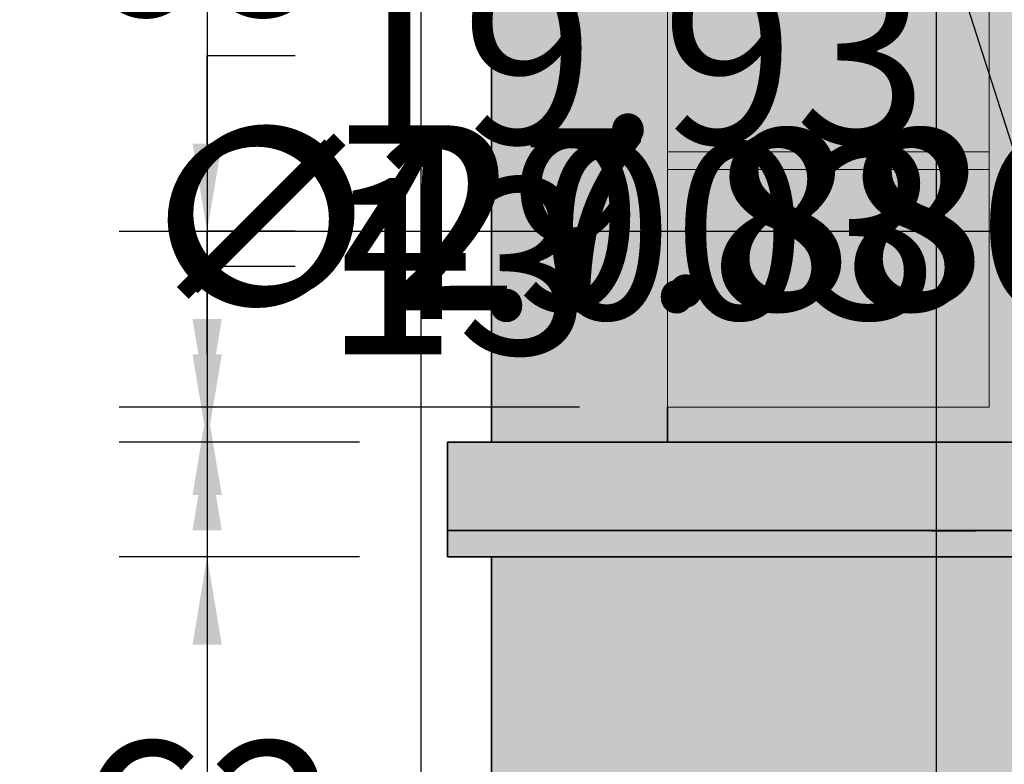
# Model space of a CAD drawing. Units: millimetres. Extents: x 130 to 1021, y 147 to 699.
# Tile 16 of 40: x 254 to 366, y 440 to 525. Entities that reach past the tile are written whole.
import ezdxf

# ---------------------------------------------------------------- set-up
doc = ezdxf.new("R2010")
doc.units = ezdxf.units.MM
doc.header["$MEASUREMENT"] = 0
for name, color, linetype, lineweight in [('A-ANNO-DIMS', 2, 'Continuous', 18), ('A-ELEV', 7, 'Continuous', 35), ('A-ELEV-PATT', 9, 'Continuous', 13), ('A-GLAZ', 4, 'Continuous', 18)]:
    doc.layers.add(name, color=color, linetype=linetype, lineweight=lineweight)
doc.styles.get("Standard").update_dxf_attribs({"font": 'arial.ttf'})
doc.dimstyles.get("Standard").update_dxf_attribs({"dimtxt": 20, "dimasz": 10, "dimexe": 10, "dimexo": 10, "dimgap": 5, "dimtad": 0, "dimtih": 1, "dimtoh": 1, "dimdec": 0, "dimzin": 0, "dimdsep": 46, "dimtxsty": 'Standard', "dimcen": 5, "dimadec": 0, "dimazin": 0, "dimtfac": 1, "dimtdec": 0, "dimtofl": 0, "dimtmove": 0, "dimatfit": 3, "dimfxl": 1, "dimtolj": 1, "dimtzin": 0, "dimarcsym": 0})

# ---------------------------------------------------------------- blocks, each defined once
blk = doc.blocks.new('*D11')
at = {"layer": 'A-ANNO-DIMS', "color": 0, "lineweight": -2, "transparency": 16777216}
for p, q in [((737.37, 648.7), (737.37, 149.74)), ((299.37, 566.95), (299.37, 149.74)), ((309.37, 159.74), (490.86, 159.74)), ((727.37, 159.74), (545.89, 159.74))]:
    blk.add_line(p, q, dxfattribs=at)
at = {"layer": 'A-ANNO-DIMS', "color": 0, "transparency": 16777216}
for points in [[(309.37, 161.41), (309.37, 158.07), (299.37, 159.74)], [(727.37, 161.41), (727.37, 158.07), (737.37, 159.74)]]:
    blk.add_solid(points, dxfattribs=at)
at = {"layer": 'Defpoints', "color": 0, "transparency": 16777216}
for p in [(737.37, 658.7), (299.37, 576.95), (737.37, 159.74)]:
    blk.add_point(p, dxfattribs=at)
at = {"layer": 'A-ANNO-DIMS', "color": 0, "transparency": 16777216, "insert": (518.37, 159.74), "char_height": 20, "attachment_point": 5}
blk.add_mtext('\\A1;438', dxfattribs=at)
blk = doc.blocks.new('*D12')
at = {"layer": 'A-ANNO-DIMS', "color": 0, "lineweight": -2, "transparency": 16777216}
for p, q in [((477.37, 661.95), (265.07, 661.95)), ((275.07, 651.95), (275.07, 438.2)), ((275.07, 194.04), (275.07, 407.78)), ((357.16, 184.04), (265.07, 184.04))]:
    blk.add_line(p, q, dxfattribs=at)
at = {"layer": 'A-ANNO-DIMS', "color": 0, "transparency": 16777216}
for points in [[(273.41, 651.95), (276.74, 651.95), (275.07, 661.95)], [(273.41, 194.04), (276.74, 194.04), (275.07, 184.04)]]:
    blk.add_solid(points, dxfattribs=at)
at = {"layer": 'Defpoints', "color": 0, "transparency": 16777216}
for p in [(275.07, 661.95), (487.37, 661.95), (367.16, 184.04)]:
    blk.add_point(p, dxfattribs=at)
at = {"layer": 'A-ANNO-DIMS', "color": 0, "transparency": 16777216, "insert": (275.07, 422.99), "char_height": 20, "attachment_point": 5}
blk.add_mtext('\\A1;477.9', dxfattribs=at)
blk = doc.blocks.new('*D15')
at = {"layer": 'A-ANNO-DIMS', "color": 0, "lineweight": -2, "transparency": 16777216}
for p, q in [((327.37, 579.88), (327.37, 696.25)), ((357.94, 411.95), (357.94, 696.25)), ((337.37, 686.25), (347.94, 686.25)), ((357.94, 686.25), (367.94, 686.25))]:
    blk.add_line(p, q, dxfattribs=at)
at = {"layer": 'A-ANNO-DIMS', "color": 0, "transparency": 16777216}
for points in [[(337.37, 687.91), (337.37, 684.58), (327.37, 686.25)], [(347.94, 687.91), (347.94, 684.58), (357.94, 686.25)]]:
    blk.add_solid(points, dxfattribs=at)
at = {"layer": 'Defpoints', "color": 0, "transparency": 16777216}
for p in [(357.94, 686.25), (327.37, 569.88), (357.94, 401.95)]:
    blk.add_point(p, dxfattribs=at)
at = {"layer": 'A-ANNO-DIMS', "color": 0, "transparency": 16777216, "insert": (406.68, 686.25), "char_height": 20, "attachment_point": 5}
blk.add_mtext('\\A1;30.57', dxfattribs=at)
blk = doc.blocks.new('*D16')
at = {"layer": 'A-ANNO-DIMS', "color": 0, "lineweight": -2, "transparency": 16777216}
for p, q in [((357.94, 411.95), (357.94, 696.25)), ((363.92, 579.88), (363.92, 696.25)), ((347.94, 686.25), (337.94, 686.25)), ((373.92, 686.25), (383.92, 686.25))]:
    blk.add_line(p, q, dxfattribs=at)
at = {"layer": 'A-ANNO-DIMS', "color": 0, "transparency": 16777216}
for points in [[(347.94, 687.91), (347.94, 684.58), (357.94, 686.25)], [(373.92, 687.91), (373.92, 684.58), (363.92, 686.25)]]:
    blk.add_solid(points, dxfattribs=at)
at = {"layer": 'Defpoints', "color": 0, "transparency": 16777216}
for p in [(363.92, 686.25), (363.92, 569.88), (357.94, 401.95)]:
    blk.add_point(p, dxfattribs=at)
at = {"layer": 'A-ANNO-DIMS', "color": 0, "transparency": 16777216, "insert": (420.74, 686.25), "char_height": 20, "attachment_point": 5}
blk.add_mtext('\\A1;5.981', dxfattribs=at)
blk = doc.blocks.new('*D17')
at = {"layer": 'A-ANNO-DIMS', "color": 0, "lineweight": -2, "transparency": 16777216}
for p, q in [((363.92, 579.88), (363.92, 696.25)), ((375.85, 490.22), (375.85, 696.25)), ((353.92, 686.25), (343.92, 686.25)), ((385.85, 686.25), (395.85, 686.25))]:
    blk.add_line(p, q, dxfattribs=at)
at = {"layer": 'A-ANNO-DIMS', "color": 0, "transparency": 16777216}
for points in [[(353.92, 687.91), (353.92, 684.58), (363.92, 686.25)], [(385.85, 687.91), (385.85, 684.58), (375.85, 686.25)]]:
    blk.add_solid(points, dxfattribs=at)
at = {"layer": 'Defpoints', "color": 0, "transparency": 16777216}
for p in [(375.85, 686.25), (363.92, 569.88), (375.85, 480.22)]:
    blk.add_point(p, dxfattribs=at)
at = {"layer": 'A-ANNO-DIMS', "color": 0, "transparency": 16777216, "insert": (441.44, 686.25), "char_height": 20, "attachment_point": 5}
blk.add_mtext('\\A1;11.928', dxfattribs=at)
blk = doc.blocks.new('*D18')
at = {"layer": 'A-ANNO-DIMS', "color": 0, "lineweight": -2, "transparency": 16777216}
for p, q in [((375.85, 490.22), (375.85, 696.25)), ((382.37, 388.95), (382.37, 696.25)), ((365.85, 686.25), (355.85, 686.25)), ((392.37, 686.25), (402.37, 686.25))]:
    blk.add_line(p, q, dxfattribs=at)
at = {"layer": 'A-ANNO-DIMS', "color": 0, "transparency": 16777216}
for points in [[(365.85, 687.91), (365.85, 684.58), (375.85, 686.25)], [(392.37, 687.91), (392.37, 684.58), (382.37, 686.25)]]:
    blk.add_solid(points, dxfattribs=at)
at = {"layer": 'Defpoints', "color": 0, "transparency": 16777216}
for p in [(382.37, 686.25), (375.85, 480.22), (382.37, 378.95)]:
    blk.add_point(p, dxfattribs=at)
at = {"layer": 'A-ANNO-DIMS', "color": 0, "transparency": 16777216, "insert": (441.13, 686.25), "char_height": 20, "attachment_point": 5}
blk.add_mtext('\\A1;6.524', dxfattribs=at)
blk = doc.blocks.new('*D40')
at = {"layer": 'A-ANNO-DIMS', "color": 0, "lineweight": -2, "transparency": 16777216}
for p, q in [((292.37, 463.95), (265.07, 463.95)), ((275.07, 453.95), (275.07, 448.16)), ((275.07, 411.95), (275.07, 417.74)), ((297.37, 401.95), (265.07, 401.95))]:
    blk.add_line(p, q, dxfattribs=at)
at = {"layer": 'A-ANNO-DIMS', "color": 0, "transparency": 16777216}
for points in [[(273.41, 453.95), (276.74, 453.95), (275.07, 463.95)], [(273.41, 411.95), (276.74, 411.95), (275.07, 401.95)]]:
    blk.add_solid(points, dxfattribs=at)
at = {"layer": 'Defpoints', "color": 0, "transparency": 16777216}
for p in [(275.07, 463.95), (302.37, 463.95), (307.37, 401.95)]:
    blk.add_point(p, dxfattribs=at)
at = {"layer": 'A-ANNO-DIMS', "color": 0, "transparency": 16777216, "insert": (275.07, 432.95), "char_height": 20, "attachment_point": 5}
blk.add_mtext('\\A1;62', dxfattribs=at)
blk = doc.blocks.new('*D41')
at = {"layer": 'A-ANNO-DIMS', "color": 0, "lineweight": -2, "transparency": 16777216}
for p, q in [((275.07, 486.95), (275.07, 496.95)), ((275.07, 496.95), (285.07, 496.95)), ((292.37, 476.95), (265.07, 476.95)), ((292.37, 463.95), (265.07, 463.95)), ((275.07, 453.95), (275.07, 443.95))]:
    blk.add_line(p, q, dxfattribs=at)
at = {"layer": 'A-ANNO-DIMS', "color": 0, "transparency": 16777216}
for points in [[(273.41, 486.95), (276.74, 486.95), (275.07, 476.95)], [(273.41, 453.95), (276.74, 453.95), (275.07, 463.95)]]:
    blk.add_solid(points, dxfattribs=at)
at = {"layer": 'Defpoints', "color": 0, "transparency": 16777216}
for p in [(275.07, 476.95), (302.37, 476.95), (302.37, 463.95)]:
    blk.add_point(p, dxfattribs=at)
at = {"layer": 'A-ANNO-DIMS', "color": 0, "transparency": 16777216, "insert": (303.46, 496.95), "char_height": 20, "attachment_point": 5}
blk.add_mtext('\\A1;13', dxfattribs=at)
blk = doc.blocks.new('*D42')
at = {"layer": 'A-ANNO-DIMS', "color": 0, "lineweight": -2, "transparency": 16777216}
for p, q in [((275.07, 490.95), (275.07, 500.95)), ((275.07, 500.95), (285.07, 500.95)), ((317.37, 480.95), (265.07, 480.95)), ((292.37, 476.95), (265.07, 476.95)), ((275.07, 466.95), (275.07, 456.95))]:
    blk.add_line(p, q, dxfattribs=at)
at = {"layer": 'A-ANNO-DIMS', "color": 0, "transparency": 16777216}
for points in [[(273.41, 490.95), (276.74, 490.95), (275.07, 480.95)], [(273.41, 466.95), (276.74, 466.95), (275.07, 476.95)]]:
    blk.add_solid(points, dxfattribs=at)
at = {"layer": 'Defpoints', "color": 0, "transparency": 16777216}
for p in [(275.07, 480.95), (327.37, 480.95), (302.37, 476.95)]:
    blk.add_point(p, dxfattribs=at)
at = {"layer": 'A-ANNO-DIMS', "color": 0, "transparency": 16777216, "insert": (324.22, 500.95), "char_height": 20, "attachment_point": 5}
blk.add_mtext('\\A1;4.003', dxfattribs=at)
blk = doc.blocks.new('*D43')
at = {"layer": 'A-ANNO-DIMS', "color": 0, "lineweight": -2, "transparency": 16777216}
for p, q in [((275.07, 510.88), (275.07, 520.88)), ((275.07, 520.88), (285.07, 520.88)), ((404.65, 500.88), (265.07, 500.88)), ((317.37, 480.95), (265.07, 480.95)), ((275.07, 470.95), (275.07, 460.95))]:
    blk.add_line(p, q, dxfattribs=at)
at = {"layer": 'A-ANNO-DIMS', "color": 0, "transparency": 16777216}
for points in [[(273.41, 510.88), (276.74, 510.88), (275.07, 500.88)], [(273.41, 470.95), (276.74, 470.95), (275.07, 480.95)]]:
    blk.add_solid(points, dxfattribs=at)
at = {"layer": 'Defpoints', "color": 0, "transparency": 16777216}
for p in [(275.07, 500.88), (414.65, 500.88), (327.37, 480.95)]:
    blk.add_point(p, dxfattribs=at)
at = {"layer": 'A-ANNO-DIMS', "color": 0, "transparency": 16777216, "insert": (322.88, 520.88), "char_height": 20, "attachment_point": 5}
blk.add_mtext('\\A1;19.93', dxfattribs=at)
blk = doc.blocks.new('*D44')
at = {"layer": 'A-ANNO-DIMS', "color": 0, "lineweight": -2, "transparency": 16777216}
for p, q in [((317.37, 569.88), (265.07, 569.88)), ((275.07, 559.88), (275.07, 550.59)), ((275.07, 510.88), (275.07, 520.17)), ((404.65, 500.88), (265.07, 500.88))]:
    blk.add_line(p, q, dxfattribs=at)
at = {"layer": 'A-ANNO-DIMS', "color": 0, "transparency": 16777216}
for points in [[(273.41, 559.88), (276.74, 559.88), (275.07, 569.88)], [(273.41, 510.88), (276.74, 510.88), (275.07, 500.88)]]:
    blk.add_solid(points, dxfattribs=at)
at = {"layer": 'Defpoints', "color": 0, "transparency": 16777216}
for p in [(275.07, 569.88), (327.37, 569.88), (414.65, 500.88)]:
    blk.add_point(p, dxfattribs=at)
at = {"layer": 'A-ANNO-DIMS', "color": 0, "transparency": 16777216, "insert": (275.07, 535.38), "char_height": 20, "attachment_point": 5}
blk.add_mtext('\\A1;69', dxfattribs=at)
blk = doc.blocks.new('*D62')
at = {"layer": 'A-ANNO-DIMS', "color": 0, "lineweight": -2, "transparency": 16777216}
for p, q in [((414.65, 495.88), (414.65, 505.88)), ((379.73, 501.93), (389.72, 501.63)), ((409.65, 500.88), (419.65, 500.88))]:
    blk.add_line(p, q, dxfattribs=at)
at = {"layer": 'A-ANNO-DIMS', "color": 0, "transparency": 16777216}
blk.add_solid([(389.77, 503.29), (389.67, 499.96), (399.72, 501.33)], dxfattribs=at)
at = {"layer": 'Defpoints', "color": 0, "transparency": 16777216}
for p in [(399.72, 501.33), (429.59, 500.43)]:
    blk.add_point(p, dxfattribs=at)
at = {"layer": 'A-ANNO-DIMS', "color": 0, "transparency": 16777216, "insert": (322.34, 501.93), "char_height": 20, "attachment_point": 5}
blk.add_mtext('\\A1;∅29.886', dxfattribs=at)
blk = doc.blocks.new('*D63')
at = {"layer": 'A-ANNO-DIMS', "color": 0, "lineweight": -2, "transparency": 16777216}
for p, q in [((414.65, 495.88), (414.65, 505.88)), ((380.75, 502.59), (390.74, 502.09)), ((409.65, 500.88), (419.65, 500.88))]:
    blk.add_line(p, q, dxfattribs=at)
at = {"layer": 'A-ANNO-DIMS', "color": 0, "transparency": 16777216}
blk.add_solid([(390.82, 503.75), (390.66, 500.42), (400.73, 501.58)], dxfattribs=at)
at = {"layer": 'Defpoints', "color": 0, "transparency": 16777216}
for p in [(400.73, 501.58), (428.58, 500.18)]:
    blk.add_point(p, dxfattribs=at)
at = {"layer": 'A-ANNO-DIMS', "color": 0, "transparency": 16777216, "insert": (323.37, 502.59), "char_height": 20, "attachment_point": 5}
blk.add_mtext('\\A1;∅27.886', dxfattribs=at)
blk = doc.blocks.new('*D64')
at = {"layer": 'A-ANNO-DIMS', "color": 0, "lineweight": -2, "transparency": 16777216}
for p, q in [((502.05, 450.93), (502.05, 460.93)), ((497.05, 455.93), (507.05, 455.93)), ((363.96, 263.06), (409.92, 327.25)), ((353.96, 263.06), (363.96, 263.06))]:
    blk.add_line(p, q, dxfattribs=at)
at = {"layer": 'A-ANNO-DIMS', "color": 0, "transparency": 16777216}
blk.add_solid([(408.57, 328.22), (411.28, 326.28), (415.74, 335.39)], dxfattribs=at)
at = {"layer": 'Defpoints', "color": 0, "transparency": 16777216}
for p in [(502.05, 455.93), (415.74, 335.39)]:
    blk.add_point(p, dxfattribs=at)
at = {"layer": 'A-ANNO-DIMS', "color": 0, "transparency": 16777216, "insert": (297.8, 263.06), "char_height": 20, "attachment_point": 5}
blk.add_mtext('\\A1;R148.25', dxfattribs=at)
blk = doc.blocks.new('*D66')
at = {"layer": 'A-ANNO-DIMS', "color": 0, "lineweight": -2, "transparency": 16777216}
for p, q in [((341.58, 557.19), (351.58, 557.19)), ((351.58, 557.19), (376.95, 478.14)), ((427.37, 315.98), (427.37, 325.98)), ((422.37, 320.98), (432.37, 320.98))]:
    blk.add_line(p, q, dxfattribs=at)
at = {"layer": 'A-ANNO-DIMS', "color": 0, "transparency": 16777216}
blk.add_solid([(378.53, 478.64), (375.36, 477.63), (380, 468.61)], dxfattribs=at)
at = {"layer": 'Defpoints', "color": 0, "transparency": 16777216}
for p in [(380, 468.61), (427.37, 320.98)]:
    blk.add_point(p, dxfattribs=at)
at = {"layer": 'A-ANNO-DIMS', "color": 0, "transparency": 16777216, "insert": (263.53, 557.19), "char_height": 20, "attachment_point": 5}
blk.add_mtext('\\A1;4X R155.05', dxfattribs=at)
blk = doc.blocks.new('*D68')
at = {"layer": 'A-ANNO-DIMS', "color": 0, "lineweight": -2, "transparency": 16777216}
for p, q in [((361.84, 579.76), (371.84, 579.76)), ((371.84, 579.76), (392.17, 506.69)), ((433.19, 354.23), (433.19, 364.23)), ((428.19, 359.23), (438.19, 359.23))]:
    blk.add_line(p, q, dxfattribs=at)
at = {"layer": 'A-ANNO-DIMS', "color": 0, "transparency": 16777216}
blk.add_solid([(393.77, 507.14), (390.56, 506.25), (394.85, 497.06)], dxfattribs=at)
at = {"layer": 'Defpoints', "color": 0, "transparency": 16777216}
for p in [(394.85, 497.06), (433.19, 359.23)]:
    blk.add_point(p, dxfattribs=at)
at = {"layer": 'A-ANNO-DIMS', "color": 0, "transparency": 16777216, "insert": (305.76, 579.76), "char_height": 20, "attachment_point": 5}
blk.add_mtext('\\A1;R143.06', dxfattribs=at)
blk = doc.blocks.new('*D70')
at = {"layer": 'A-ANNO-DIMS', "color": 0, "lineweight": -2, "transparency": 16777216}
for p, q in [((370.14, 588.4), (380.14, 588.4)), ((380.14, 588.4), (397.47, 517.01)), ((432.65, 367.11), (432.65, 377.11)), ((427.65, 372.11), (437.65, 372.11))]:
    blk.add_line(p, q, dxfattribs=at)
at = {"layer": 'A-ANNO-DIMS', "color": 0, "transparency": 16777216}
blk.add_solid([(399.09, 517.4), (395.85, 516.62), (399.83, 507.29)], dxfattribs=at)
at = {"layer": 'Defpoints', "color": 0, "transparency": 16777216}
for p in [(399.83, 507.29), (432.65, 372.11)]:
    blk.add_point(p, dxfattribs=at)
at = {"layer": 'A-ANNO-DIMS', "color": 0, "transparency": 16777216, "insert": (323.76, 588.4), "char_height": 20, "attachment_point": 5}
blk.add_mtext('\\A1;R139.1', dxfattribs=at)
blk = doc.blocks.new('*D73')
at = {"layer": 'A-ANNO-DIMS', "color": 0, "lineweight": -2, "transparency": 16777216}
for p, q in [((402.68, 571.45), (412.68, 571.45)), ((412.68, 571.45), (419.05, 502.17)), ((432.11, 355.14), (432.11, 365.14)), ((427.11, 360.14), (437.11, 360.14))]:
    blk.add_line(p, q, dxfattribs=at)
at = {"layer": 'A-ANNO-DIMS', "color": 0, "transparency": 16777216}
blk.add_solid([(420.71, 502.32), (417.39, 502.01), (419.97, 492.21)], dxfattribs=at)
at = {"layer": 'Defpoints', "color": 0, "transparency": 16777216}
for p in [(419.97, 492.21), (432.11, 360.14)]:
    blk.add_point(p, dxfattribs=at)
at = {"layer": 'A-ANNO-DIMS', "color": 0, "transparency": 16777216, "insert": (346.7, 571.45), "char_height": 20, "attachment_point": 5}
blk.add_mtext('\\A1;R132.62', dxfattribs=at)

msp = doc.modelspace()

# ---------------------------------------------------------------- hatches: boundary and pattern name
at = {"layer": 'A-ELEV-PATT'}
h = msp.add_hatch(color=256, dxfattribs=at)
h.dxf.hatch_style = 1
h.paths.add_polyline_path([(737.3738, 658.6988, 0.01359606), (632.4019, 661.9473), (607.3738, 661.9473), (487.3738, 661.9473), (487.3738, 649.9473), (607.3738, 649.9473), (632.3794, 649.9473, -0.01368411), (737.3738, 646.6784)])
h.paths.add_polyline_path([(732.3738, 643.9599, 0.01305286), (632.3738, 646.9473), (607.3738, 646.9473), (487.3738, 646.9473), (487.3738, 596.9473), (632.3738, 596.9473, -0.01305286), (732.3738, 593.9599)])
h.paths.add_polyline_path([(737.3738, 593.6732, 0.01370629), (632.3738, 596.9473), (487.3738, 596.9473), (487.3738, 586.9473), (632.355, 586.9473, -0.01378075), (737.3738, 583.6559)])
h.paths.add_polyline_path([(447.3738, 646.9473), (307.3738, 646.9473), (302.3738, 646.9473), (302.3738, 634.9473), (447.3738, 634.9473)])
h.paths.add_polyline_path([(447.3738, 631.9473), (307.3738, 631.9473), (307.3738, 586.9473), (447.3738, 586.9473)])
h.paths.add_polyline_path([(447.3738, 586.9473), (307.3738, 586.9473), (302.3738, 586.9473), (302.3738, 576.9473), (447.3738, 576.9473)])
h.paths.add_polyline_path([(447.3738, 573.9473), (367.3738, 573.9473), (367.3738, 539.9473), (447.3738, 539.9473)])
h.paths.add_polyline_path([(447.3738, 537.9473), (367.3738, 537.9473), (367.3738, 507.9473), (400.392, 507.4253, -0.00172798), (401.3281, 507.6451, -0.52200255), (425.6117, 511.0391, -0.03918489), (447.3738, 510.4359), (447.3738, 510.7883)])
h.paths.add_polyline_path([(394.7238, 505.9473), (367.3738, 505.9473), (367.3738, 476.9473, -0.0146512), (375.8501, 480.2159), (376.1506, 499.2266, -0.03554194)])
h.paths.add_polyline_path([(632.3738, 583.9473), (552.3738, 583.9473), (552.3738, 550.9473), (632.3738, 550.9473)])
h.paths.add_polyline_path([(632.3738, 548.9473), (552.3738, 548.9473), (552.3738, 515.9473), (632.3738, 515.9473)])
h.paths.add_polyline_path([(632.3738, 513.9473), (552.3738, 513.9473), (552.3738, 476.9473), (632.3738, 476.9473)])
h.paths.add_polyline_path([(737.3738, 473.6903, 0.01363261), (632.3926, 476.9473), (552.3738, 476.9473), (487.3738, 476.9473), (487.3738, 466.9473), (632.3738, 466.9473, -0.01370629), (737.3738, 463.6732)])
h.paths.add_polyline_path([(732.3738, 460.9552, 0.01307409), (632.3681, 463.9473), (487.3738, 463.9473), (487.3738, 407.735, -0.00322862), (489.3544, 406.9473), (632.3926, 406.9473, -0.01298259), (732.3738, 403.9755)])
h.paths.add_polyline_path([(487.3738, 463.9473, 0.20132998), (367.3738, 463.9473), (367.3738, 407.735, -0.18820307), (487.3738, 407.735)])
h.paths.add_polyline_path([(367.3738, 476.9473), (367.3738, 466.9473, -0.20133085), (487.3738, 466.9473), (487.3738, 476.9473, 0.20132998)])
h.paths.add_polyline_path([(367.3738, 463.9473), (307.3738, 463.9473), (307.3738, 401.9473), (357.9413, 401.9473), (367.3738, 407.735)])
h.paths.add_polyline_path([(367.3738, 476.9473), (302.3738, 476.9473), (302.3738, 466.9473), (367.3738, 466.9473)])
h.paths.add_polyline_path([(632.8184, 366.9453), (552.3738, 366.9453), (552.3738, 393.9473), (632.8184, 393.9473)])
h.paths.add_polyline_path([(632.8184, 357.2114), (632.8184, 363.9453), (552.3738, 363.9453), (552.3738, 357.2114), (552.3738, 336.9453), (632.8184, 336.9453)])
h.paths.add_polyline_path([(632.8184, 333.9453), (552.3738, 333.9453), (552.3738, 306.9453), (632.8184, 306.9453)])
h.paths.add_polyline_path([(632.8184, 303.9453), (552.3738, 303.9453), (552.3738, 273.9473), (632.355, 273.9473, 0.00006077), (632.8184, 273.9491)])
h.paths.add_polyline_path([(737.3738, 403.6903, 0.01363261), (632.3926, 406.9473), (489.3544, 406.9473, 0.19154808), (367.3738, 407.735), (367.3738, 396.9473, -0.20133085), (487.3738, 396.9473), (632.3738, 396.9473, -0.01370629), (737.3738, 393.6732)])
h.paths.add_polyline_path([(357.9413, 401.9473), (307.3738, 401.9473), (307.3738, 391.9473), (357.9413, 391.9473)])
h.paths.add_polyline_path([(357.9413, 357.2114), (357.9413, 388.9473), (307.3738, 388.9473), (307.3738, 357.2114), (307.3738, 273.9473), (357.9413, 273.9473)])
h.paths.add_polyline_path([(732.3738, 263.93, -0.0130317), (632.3794, 260.9473), (466.7667, 260.9473), (466.7667, 240.9473), (469.8406, 236.978), (469.8406, 221.978), (472.9145, 218.0087), (472.9145, 213.9473), (607.3738, 213.9473), (732.3738, 213.9473)])
h.paths.add_polyline_path([(732.3738, 290.889), (722.479, 290.889), (722.479, 301.889), (732.3738, 301.889), (732.3738, 305.889), (722.479, 305.889), (722.479, 316.889), (732.3738, 316.889), (732.3738, 320.889), (722.479, 320.889), (722.479, 331.889), (732.3738, 331.889), (732.3738, 335.889), (722.479, 335.889), (722.479, 346.889), (732.3738, 346.889), (732.3738, 350.889), (722.479, 350.889), (722.479, 361.889), (732.3738, 361.889), (732.3738, 365.889), (722.479, 365.889), (722.479, 376.889), (732.3738, 376.889), (732.3738, 380.889), (722.479, 380.889), (722.479, 391.4848, 0.00052326), (718.479, 391.6843), (718.479, 380.889), (707.479, 380.889), (707.479, 392.1896, 0.00052307), (703.479, 392.3576), (703.479, 380.889), (692.479, 380.889), (692.479, 392.7765, 0.00052292), (688.479, 392.9131), (688.479, 380.889), (677.479, 380.889), (677.479, 393.2456, 0.00052279), (673.479, 393.3508), (673.479, 380.889), (662.479, 380.889), (662.479, 393.597, 0.0005227), (658.479, 393.6709), (658.479, 380.889), (647.479, 380.889), (647.479, 393.8308, 0.00052264), (643.479, 393.8732), (643.479, 380.889), (632.8184, 380.889), (632.8184, 376.889), (643.479, 376.889), (643.479, 365.889), (632.8184, 365.889), (632.8184, 361.889), (643.479, 361.889), (643.479, 350.889), (632.8184, 350.889), (632.8184, 346.889), (643.479, 346.889), (643.479, 335.889), (632.8184, 335.889), (632.8184, 331.889), (643.479, 331.889), (643.479, 320.889), (632.8184, 320.889), (632.8184, 316.889), (643.479, 316.889), (643.479, 305.889), (632.8184, 305.889), (632.8184, 301.889), (643.479, 301.889), (643.479, 290.889), (632.8184, 290.889), (632.8184, 286.889), (643.479, 286.889), (643.479, 274.0217, 0.00052456), (647.479, 274.0643), (647.479, 286.889), (658.479, 286.889), (658.479, 274.2248, 0.00052462), (662.479, 274.2989), (662.479, 286.889), (673.479, 286.889), (673.479, 274.546, 0.00052471), (677.479, 274.6516), (677.479, 286.889), (688.479, 286.889), (688.479, 274.9853, 0.00052484), (692.479, 275.1224), (692.479, 286.889), (703.479, 286.889), (703.479, 275.5429, 0.000525), (707.479, 275.7115), (707.479, 286.889), (718.479, 286.889), (718.479, 276.2187, 0.00052519), (722.479, 276.4189), (722.479, 286.889), (732.3738, 286.889)])
h.paths.add_polyline_path([(718.479, 290.889), (707.479, 290.889), (707.479, 301.889), (718.479, 301.889)], flags=16)
h.paths.add_polyline_path([(703.479, 290.889), (692.479, 290.889), (692.479, 301.889), (703.479, 301.889)], flags=16)
h.paths.add_polyline_path([(718.479, 305.889), (707.479, 305.889), (707.479, 316.889), (718.479, 316.889)], flags=16)
h.paths.add_polyline_path([(703.479, 305.889), (692.479, 305.889), (692.479, 316.889), (703.479, 316.889)], flags=16)
h.paths.add_polyline_path([(688.479, 290.889), (677.479, 290.889), (677.479, 301.889), (688.479, 301.889)], flags=16)
h.paths.add_polyline_path([(718.479, 320.889), (707.479, 320.889), (707.479, 331.889), (718.479, 331.889)], flags=16)
h.paths.add_polyline_path([(688.479, 305.889), (677.479, 305.889), (677.479, 316.889), (688.479, 316.889)], flags=16)
h.paths.add_polyline_path([(703.479, 320.889), (692.479, 320.889), (692.479, 331.889), (703.479, 331.889)], flags=16)
h.paths.add_polyline_path([(688.479, 320.889), (677.479, 320.889), (677.479, 331.889), (688.479, 331.889)], flags=16)
h.paths.add_polyline_path([(673.479, 290.889), (662.479, 290.889), (662.479, 301.889), (673.479, 301.889)], flags=16)
h.paths.add_polyline_path([(718.479, 335.889), (707.479, 335.889), (707.479, 346.889), (718.479, 346.889)], flags=16)
h.paths.add_polyline_path([(673.479, 305.889), (662.479, 305.889), (662.479, 316.889), (673.479, 316.889)], flags=16)
h.paths.add_polyline_path([(703.479, 335.889), (692.479, 335.889), (692.479, 346.889), (703.479, 346.889)], flags=16)
h.paths.add_polyline_path([(673.479, 320.889), (662.479, 320.889), (662.479, 331.889), (673.479, 331.889)], flags=16)
h.paths.add_polyline_path([(688.479, 335.889), (677.479, 335.889), (677.479, 346.889), (688.479, 346.889)], flags=16)
h.paths.add_polyline_path([(658.479, 290.889), (647.479, 290.889), (647.479, 301.889), (658.479, 301.889)], flags=16)
h.paths.add_polyline_path([(718.479, 350.889), (707.479, 350.889), (707.479, 361.889), (718.479, 361.889)], flags=16)
h.paths.add_polyline_path([(658.479, 305.889), (647.479, 305.889), (647.479, 316.889), (658.479, 316.889)], flags=16)
h.paths.add_polyline_path([(703.479, 350.889), (692.479, 350.889), (692.479, 361.889), (703.479, 361.889)], flags=16)
h.paths.add_polyline_path([(673.479, 335.889), (662.479, 335.889), (662.479, 346.889), (673.479, 346.889)], flags=16)
h.paths.add_polyline_path([(658.479, 320.889), (647.479, 320.889), (647.479, 331.889), (658.479, 331.889)], flags=16)
h.paths.add_polyline_path([(688.479, 350.889), (677.479, 350.889), (677.479, 361.889), (688.479, 361.889)], flags=16)
h.paths.add_polyline_path([(718.479, 365.889), (707.479, 365.889), (707.479, 376.889), (718.479, 376.889)], flags=16)
h.paths.add_polyline_path([(658.479, 335.889), (647.479, 335.889), (647.479, 346.889), (658.479, 346.889)], flags=16)
h.paths.add_polyline_path([(673.479, 350.889), (662.479, 350.889), (662.479, 361.889), (673.479, 361.889)], flags=16)
h.paths.add_polyline_path([(703.479, 365.889), (692.479, 365.889), (692.479, 376.889), (703.479, 376.889)], flags=16)
h.paths.add_polyline_path([(688.479, 365.889), (677.479, 365.889), (677.479, 376.889), (688.479, 376.889)], flags=16)
h.paths.add_polyline_path([(658.479, 350.889), (647.479, 350.889), (647.479, 361.889), (658.479, 361.889)], flags=16)
h.paths.add_polyline_path([(673.479, 365.889), (662.479, 365.889), (662.479, 376.889), (673.479, 376.889)], flags=16)
h.paths.add_polyline_path([(658.479, 365.889), (647.479, 365.889), (647.479, 376.889), (658.479, 376.889)], flags=16)
h.paths.add_polyline_path([(732.3738, 503.9786), (722.3392, 503.9786), (722.3392, 514.9786), (732.3738, 514.9786), (732.3738, 518.9786), (722.3392, 518.9786), (722.3392, 529.9786), (732.3738, 529.9786), (732.3738, 533.9786), (722.3392, 533.9786), (722.3392, 544.9786), (732.3738, 544.9786), (732.3738, 546.9473), (732.3738, 548.9786), (722.3392, 548.9786), (722.3392, 559.9786), (732.3738, 559.9786), (732.3738, 563.9786), (722.3392, 563.9786), (722.3392, 574.9786), (732.3738, 574.9786), (732.3738, 578.9786), (722.3392, 578.9786), (722.3392, 581.4789, 0.00052601), (718.3392, 581.6791), (718.3392, 578.9786), (707.3392, 578.9786), (707.3392, 582.1863, 0.00052582), (703.3392, 582.355), (703.3392, 578.9786), (692.3392, 578.9786), (692.3392, 582.7752, 0.00052566), (688.3392, 582.9123), (688.3392, 578.9786), (677.3392, 578.9786), (677.3392, 583.2457, 0.00052554), (673.3392, 583.3512), (673.3392, 578.9786), (662.3392, 578.9786), (662.3392, 583.5978, 0.00052545), (658.3392, 583.6718), (658.3392, 578.9786), (647.3392, 578.9786), (647.3392, 583.8317, 0.00052539), (643.3392, 583.8741), (643.3392, 578.9786), (632.3738, 578.9786), (632.3738, 574.9786), (643.3392, 574.9786), (643.3392, 563.9786), (632.3738, 563.9786), (632.3738, 559.9786), (643.3392, 559.9786), (643.3392, 548.9786), (632.3738, 548.9786), (632.3738, 544.9786), (643.3392, 544.9786), (643.3392, 533.9786), (632.3738, 533.9786), (632.3738, 529.9786), (643.3392, 529.9786), (643.3392, 518.9786), (632.3738, 518.9786), (632.3738, 515.9473), (632.3738, 514.9786), (643.3392, 514.9786), (643.3392, 503.9786), (632.3738, 503.9786), (632.3738, 499.9786), (643.3392, 499.9786), (643.3392, 488.9786), (632.3738, 488.9786), (632.3738, 484.9786), (643.3392, 484.9786), (643.3392, 476.8751, -0.00051911), (647.3392, 476.8332), (647.3392, 484.9786), (658.3392, 484.9786), (658.3392, 476.6752, -0.00051917), (662.3392, 476.6022), (662.3392, 484.9786), (673.3392, 484.9786), (673.3392, 476.3585, -0.00051926), (677.3392, 476.2543), (677.3392, 484.9786), (688.3392, 484.9786), (688.3392, 475.9248, -0.00051938), (692.3392, 475.7894), (692.3392, 484.9786), (703.3392, 484.9786), (703.3392, 475.3741, -0.00051953), (707.3392, 475.2075), (707.3392, 484.9786), (718.3392, 484.9786), (718.3392, 474.7064, -0.00051972), (722.3392, 474.5086), (722.3392, 484.9786), (732.3738, 484.9786), (732.3738, 488.9786), (722.3392, 488.9786), (722.3392, 499.9786), (732.3738, 499.9786)])
h.paths.add_polyline_path([(718.3392, 503.9786), (707.3392, 503.9786), (707.3392, 514.9786), (718.3392, 514.9786)], flags=16)
h.paths.add_polyline_path([(718.3392, 499.9786), (718.3392, 488.9786), (707.3392, 488.9786), (707.3392, 499.9786)], flags=16)
h.paths.add_polyline_path([(718.3392, 518.9786), (707.3392, 518.9786), (707.3392, 529.9786), (718.3392, 529.9786)], flags=16)
h.paths.add_polyline_path([(703.3392, 503.9786), (692.3392, 503.9786), (692.3392, 514.9786), (703.3392, 514.9786)], flags=16)
h.paths.add_polyline_path([(703.3392, 499.9786), (703.3392, 488.9786), (692.3392, 488.9786), (692.3392, 499.9786)], flags=16)
h.paths.add_polyline_path([(703.3392, 518.9786), (692.3392, 518.9786), (692.3392, 529.9786), (703.3392, 529.9786)], flags=16)
h.paths.add_polyline_path([(718.3392, 533.9786), (707.3392, 533.9786), (707.3392, 544.9786), (718.3392, 544.9786)], flags=16)
h.paths.add_polyline_path([(688.3392, 503.9786), (677.3392, 503.9786), (677.3392, 514.9786), (688.3392, 514.9786)], flags=16)
h.paths.add_polyline_path([(688.3392, 499.9786), (688.3392, 488.9786), (677.3392, 488.9786), (677.3392, 499.9786)], flags=16)
h.paths.add_polyline_path([(703.3392, 533.9786), (692.3392, 533.9786), (692.3392, 544.9786), (703.3392, 544.9786)], flags=16)
h.paths.add_polyline_path([(688.3392, 518.9786), (677.3392, 518.9786), (677.3392, 529.9786), (688.3392, 529.9786)], flags=16)
h.paths.add_polyline_path([(688.3392, 533.9786), (677.3392, 533.9786), (677.3392, 544.9786), (688.3392, 544.9786)], flags=16)
h.paths.add_polyline_path([(718.3392, 548.9786), (707.3392, 548.9786), (707.3392, 559.9786), (718.3392, 559.9786)], flags=16)
h.paths.add_polyline_path([(673.3392, 503.9786), (662.3392, 503.9786), (662.3392, 514.9786), (673.3392, 514.9786)], flags=16)
h.paths.add_polyline_path([(673.3392, 499.9786), (673.3392, 488.9786), (662.3392, 488.9786), (662.3392, 499.9786)], flags=16)
h.paths.add_polyline_path([(703.3392, 548.9786), (692.3392, 548.9786), (692.3392, 559.9786), (703.3392, 559.9786)], flags=16)
h.paths.add_polyline_path([(673.3392, 518.9786), (662.3392, 518.9786), (662.3392, 529.9786), (673.3392, 529.9786)], flags=16)
h.paths.add_polyline_path([(688.3392, 548.9786), (677.3392, 548.9786), (677.3392, 559.9786), (688.3392, 559.9786)], flags=16)
h.paths.add_polyline_path([(673.3392, 533.9786), (662.3392, 533.9786), (662.3392, 544.9786), (673.3392, 544.9786)], flags=16)
h.paths.add_polyline_path([(718.3392, 563.9786), (707.3392, 563.9786), (707.3392, 574.9786), (718.3392, 574.9786)], flags=16)
h.paths.add_polyline_path([(658.3392, 503.9786), (647.3392, 503.9786), (647.3392, 514.9786), (658.3392, 514.9786)], flags=16)
h.paths.add_polyline_path([(658.3392, 499.9786), (658.3392, 488.9786), (647.3392, 488.9786), (647.3392, 499.9786)], flags=16)
h.paths.add_polyline_path([(703.3392, 563.9786), (692.3392, 563.9786), (692.3392, 574.9786), (703.3392, 574.9786)], flags=16)
h.paths.add_polyline_path([(658.3392, 518.9786), (647.3392, 518.9786), (647.3392, 529.9786), (658.3392, 529.9786)], flags=16)
h.paths.add_polyline_path([(673.3392, 548.9786), (662.3392, 548.9786), (662.3392, 559.9786), (673.3392, 559.9786)], flags=16)
h.paths.add_polyline_path([(688.3392, 563.9786), (677.3392, 563.9786), (677.3392, 574.9786), (688.3392, 574.9786)], flags=16)
h.paths.add_polyline_path([(658.3392, 533.9786), (647.3392, 533.9786), (647.3392, 544.9786), (658.3392, 544.9786)], flags=16)
h.paths.add_polyline_path([(673.3392, 563.9786), (662.3392, 563.9786), (662.3392, 574.9786), (673.3392, 574.9786)], flags=16)
h.paths.add_polyline_path([(658.3392, 548.9786), (647.3392, 548.9786), (647.3392, 559.9786), (658.3392, 559.9786)], flags=16)
h.paths.add_polyline_path([(658.3392, 563.9786), (647.3392, 563.9786), (647.3392, 574.9786), (658.3392, 574.9786)], flags=16)
h = msp.add_hatch(color=256, dxfattribs=at)
h.dxf.hatch_style = 1
h.paths.add_polyline_path([(447.3738, 576.9473), (302.3738, 576.9473), (302.3738, 573.9473), (447.3738, 573.9473)])
h.paths.add_polyline_path([(487.3738, 583.9473), (487.3738, 586.9473), (447.3738, 576.9473), (447.3738, 573.9473)])
h.paths.add_polyline_path([(632.355, 586.9473), (487.3738, 586.9473), (487.3738, 583.9473), (632.3738, 583.9473), (632.3738, 583.9472, -0.01380003), (737.3738, 580.6507), (737.3738, 583.6559, 0.01378075)])
h.paths.add_polyline_path([(367.3738, 466.9473), (302.3738, 466.9473), (302.3738, 463.9473), (367.3738, 463.9473)])
h.paths.add_polyline_path([(487.3738, 463.9473), (487.3738, 466.9473, 0.20133085), (367.3738, 466.9473), (367.3738, 463.9473, -0.20132998)])
h.paths.add_polyline_path([(632.3738, 466.9473), (487.3738, 466.9473), (487.3738, 463.9473), (632.3681, 463.9473, -0.01372855), (737.3738, 460.6681), (737.3738, 463.6732, 0.01370629)])
h.paths.add_polyline_path([(632.3738, 396.9473), (487.3738, 396.9473, 0.20133085), (367.3738, 396.9473), (367.3738, 393.9473, -0.20237172), (486.7667, 393.9473), (632.3681, 393.9473, -0.01372855), (737.3738, 390.6681), (737.3738, 393.6732, 0.01370629)])
h.paths.add_polyline_path([(357.9413, 391.9473), (307.3738, 391.9473), (307.3738, 388.9473), (357.9413, 388.9473)])
h.paths.add_polyline_path([(367.3738, 393.9473), (367.3738, 396.9473), (357.9413, 391.924), (357.9413, 388.9473), (358.058, 388.9473)])
h.paths.add_polyline_path([(737.3738, 264.2162), (737.3738, 267.2214, -0.01370629), (632.3738, 263.9473), (463.7667, 263.9473), (466.7667, 260.9473), (632.3794, 260.9473, 0.01368411)])
h.paths.add_polyline_path([(463.7667, 263.9473), (447.3738, 263.9473), (450.3738, 260.9473), (466.7667, 260.9473)])
h.paths.add_polyline_path([(447.3738, 263.9473), (432.3738, 263.9473), (432.3738, 260.9473), (450.3738, 260.9473)])
h.paths.add_polyline_path([(382.3738, 263.9473), (357.9413, 263.9473), (357.9413, 260.9473), (382.3738, 260.9473)])
h.paths.add_polyline_path([(357.9413, 263.9473), (307.3738, 263.9473), (307.3738, 260.9473), (357.9413, 260.9473)])
h = msp.add_hatch(color=256, dxfattribs=at)
h.paths.add_polyline_path([(327.3738, 569.884), (327.3738, 573.9473), (307.3738, 573.9473), (307.3738, 476.9473), (327.3738, 476.9473), (327.3738, 480.95)])
h.paths.add_polyline_path([(486.7667, 386.2639), (486.7667, 393.9473), (466.7667, 393.9473), (466.7667, 357.2114), (466.7667, 311.9335, 0.03427026), (486.7667, 308.4637)])
h.paths.add_polyline_path([(486.7667, 308.4637, -0.03427026), (466.7667, 311.9335), (466.7667, 273.9473), (486.7667, 273.9473)])
h.paths.add_polyline_path([(389.3738, 351.5473), (396.7693, 351.5473, -0.00702703), (393.8774, 354.5473), (389.3738, 354.5473), (389.3738, 359.5775, -0.01903024), (382.3738, 368.424), (382.3738, 249.5473), (432.3738, 249.5473), (432.3738, 325.067, -0.00576734), (429.3738, 326.709), (429.3738, 257.5473), (426.3738, 257.5473), (426.3738, 328.4428, -0.00592542), (423.3738, 330.272), (423.3738, 315.7473), (389.3738, 315.7473), (389.3738, 332.1473), (420.4552, 332.1473, -0.00895099), (416.0768, 335.1473), (389.3738, 335.1473)])
h.paths.add_polyline_path([(389.3738, 312.7473), (423.3738, 312.7473), (423.3738, 296.3473), (389.3738, 296.3473)], flags=16)
h.paths.add_polyline_path([(389.3738, 293.3473), (423.3738, 293.3473), (423.3738, 276.9473), (389.3738, 276.9473)], flags=16)
h.paths.add_polyline_path([(389.3738, 273.9473), (423.3738, 273.9473), (423.3738, 257.5473), (389.3738, 257.5473)], flags=16)
h.paths.add_polyline_path([(432.3738, 378.9473), (382.3738, 378.9473), (382.3738, 368.424, 0.01903024), (389.3738, 359.5775), (389.3738, 370.9473), (423.3738, 370.9473), (423.3738, 354.5473), (393.8774, 354.5473, 0.00702703), (396.7693, 351.5473), (423.3738, 351.5473), (423.3738, 335.1473), (416.0768, 335.1473, 0.00895099), (420.4552, 332.1473), (423.3738, 332.1473), (423.3738, 330.272, 0.00592542), (426.3738, 328.4428), (426.3738, 370.9473), (429.3738, 370.9473), (429.3738, 326.709, 0.00576734), (432.3738, 325.067)])
h.paths.add_polyline_path([(466.7667, 357.2114), (466.7667, 393.9473), (447.3738, 393.9473), (447.3738, 357.2114), (447.3738, 318.1243, 0.0063261), (450.8779, 316.785), (450.8779, 331.5915), (463.5608, 331.5915), (463.5608, 312.7571, 0.00558197), (466.7667, 311.9335)])
h.paths.add_polyline_path([(450.8779, 334.5915), (450.8779, 360.0915), (463.5608, 360.0915), (463.5608, 334.5915)], flags=16)
h.paths.add_polyline_path([(450.8779, 363.0915), (450.8779, 388.6449), (463.5608, 388.6449), (463.5608, 363.0915)], flags=16)
h.paths.add_polyline_path([(466.7667, 311.9335, -0.00558197), (463.5608, 312.7571), (463.5608, 306.0915), (450.8779, 306.0915), (450.8779, 316.785, -0.0063261), (447.3738, 318.1243), (447.3738, 273.9473), (466.7667, 273.9473)])
h.paths.add_polyline_path([(450.8779, 303.0915), (463.5608, 303.0915), (463.5608, 277.5915), (450.8779, 277.5915)], flags=16)
h.paths.add_polyline_path([(552.3738, 357.2114), (552.3738, 393.9473), (486.7667, 393.9473), (486.7667, 386.2639), (544.6354, 386.2639), (544.6354, 280.6619), (486.7667, 280.6619), (486.7667, 273.9473), (552.3738, 273.9473)])
h.paths.add_polyline_path([(487.3738, 583.9473), (472.3738, 580.1973), (472.3738, 507.0765), (472.3738, 505.4251, -0.00564525), (475.3738, 504.4942), (475.3738, 506.3543), (475.3738, 511.9473), (484.3738, 511.9473), (484.3738, 503.8134), (484.3738, 501.2439, -0.00583574), (487.3738, 500.0015)])
h.paths.add_polyline_path([(484.3738, 578.0434), (484.3738, 548.9473), (475.3738, 548.9473), (475.3738, 575.7934)], flags=16)
h.paths.add_polyline_path([(484.3738, 546.9473), (484.3738, 513.9473), (475.3738, 513.9473), (475.3738, 518.7148), (475.3738, 546.9473)], flags=16)
msp.add_hatch(color=256, dxfattribs=at).paths.add_polyline_path([(327.3738, 573.9473), (327.3738, 569.884), (363.922, 569.884), (363.922, 480.95), (327.3738, 480.95), (327.3738, 476.9473), (367.3738, 476.9473), (367.3738, 573.9473)])
h = msp.add_hatch(color=256, dxfattribs=at)
h.paths.add_polyline_path([(327.3738, 541.9473), (327.3738, 539.9473), (363.922, 539.9473), (363.922, 541.9473)])
h.paths.add_polyline_path([(327.3738, 509.9473), (327.3738, 507.9473), (363.922, 507.9473), (363.922, 509.9473)])
h = msp.add_hatch(color=256, dxfattribs=at)
h.dxf.hatch_style = 1
h.paths.add_polyline_path([(364.0891, 218.0087), (361.0152, 221.978), (361.0152, 236.978), (357.9413, 240.9473), (357.9413, 195.9473), (367.163, 184.0395), (367.163, 199.0395), (364.0891, 203.0087)])
h.paths.add_polyline_path([(502.3738, 537.2685), (502.3738, 513.9473), (547.7773, 513.9473), (547.7773, 537.2685)])
h.paths.add_polyline_path([(502.3738, 511.9473), (502.3738, 481.7432), (547.7773, 481.7432), (547.7773, 511.9473)])
h.paths.add_polyline_path([(327.3738, 529.7), (327.3738, 509.9473), (363.922, 509.9473), (363.922, 529.7)])
h.paths.add_polyline_path([(327.3738, 507.9473), (327.3738, 480.95), (363.922, 480.95), (363.922, 507.9473)])

# ---------------------------------------------------------------- linework, layer by layer
at = {"layer": 'A-ELEV'}
for p, q in [((307.3738, 573.9473), (307.3738, 476.9473)), ((327.3738, 480.95), (327.3738, 476.9473)), ((302.3738, 476.9473), (302.3738, 463.9473)), ((367.3738, 476.9473), (302.3738, 476.9473)), ((367.3738, 466.9473), (302.3738, 466.9473)), ((367.3738, 466.9473), (357.3742, 466.8599)), ((367.3738, 463.9473), (302.3738, 463.9473)), ((307.3738, 463.9473), (307.3738, 357.2114))]:
    msp.add_line(p, q, dxfattribs=at)
at = {"layer": 'A-GLAZ'}
for p, q in [((363.922, 509.9473), (327.3738, 509.9473)), ((363.922, 507.9473), (327.3738, 507.9473))]:
    msp.add_line(p, q, dxfattribs=at)
msp.add_lwpolyline([(363.922, 569.884), (327.3738, 569.884), (327.3738, 480.95), (363.922, 480.95)], close=True, dxfattribs=at)

# ---------------------------------------------------------------- dimensions: what is measured, and where the dimension line sits
at = {"layer": 'A-ANNO-DIMS'}
for base, p1, p2, override, picture, middle in [((357.9413, 686.2473), (327.3738, 569.884), (357.9413, 401.9473), {"dimdec": 2, "dimlfac": 1, "dimrnd": 0, "dimzin": 0, "dimdsep": 46, "dimlunit": 2}, '*D15', (406.6794, 686.2473)), ((363.922, 686.2473), (357.9413, 401.9473), (363.922, 569.884), {"dimdec": 3, "dimlfac": 1, "dimrnd": 0, "dimzin": 0, "dimdsep": 46, "dimlunit": 2}, '*D16', (420.7365, 686.2473)), ((375.8501, 686.2473), (363.922, 569.884), (375.8501, 480.2159), {"dimdec": 3, "dimlfac": 1, "dimrnd": 0, "dimzin": 0, "dimdsep": 46, "dimlunit": 2}, '*D17', (441.4435, 686.2473)), ((382.3738, 686.2473), (375.8501, 480.2159), (382.3738, 378.9473), {"dimdec": 3, "dimlfac": 1, "dimrnd": 0, "dimzin": 0, "dimdsep": 46, "dimlunit": 2}, '*D18', (441.1323, 686.2473)), ((737.3738, 159.7395), (299.3738, 576.9473), (737.3738, 658.6988), {"dimdec": 0, "dimlfac": 1, "dimrnd": 0, "dimzin": 0, "dimdsep": 46, "dimlunit": 2}, '*D11', (518.3738, 159.7395))]:
    dim = msp.add_linear_dim(base=base, p1=p1, p2=p2, dimstyle='Standard', override=override, dxfattribs=at)
    dim.commit()
    dim.dimension.update_dxf_attribs({"geometry": picture, "text_midpoint": middle})
for base, p1, p2, override, picture, middle in [((275.0738, 661.9473), (367.163, 184.0395), (487.3738, 661.9473), {"dimdec": 1, "dimlfac": 1, "dimrnd": 0, "dimzin": 0, "dimdsep": 46, "dimlunit": 2}, '*D12', (275.0738, 422.9934)), ((275.0738, 569.884), (414.6525, 500.8811), (327.3738, 569.884), {"dimdec": 0, "dimlfac": 1, "dimrnd": 0, "dimzin": 0, "dimdsep": 46, "dimlunit": 2}, '*D44', (275.0738, 535.3826)), ((275.0738, 500.8811), (327.3738, 480.95), (414.6525, 500.8811), {"dimdec": 2, "dimlfac": 1, "dimrnd": 0, "dimzin": 0, "dimdsep": 46, "dimlunit": 2}, '*D43', (322.8773, 520.8811)), ((275.0738, 480.95), (302.3738, 476.9473), (327.3738, 480.95), {"dimdec": 3, "dimlfac": 1, "dimrnd": 0, "dimzin": 0, "dimdsep": 46, "dimlunit": 2}, '*D42', (324.2211, 500.95)), ((275.0738, 476.9473), (302.3738, 463.9473), (302.3738, 476.9473), {"dimdec": 0, "dimlfac": 1, "dimrnd": 0, "dimzin": 0, "dimdsep": 46, "dimlunit": 2}, '*D41', (303.4571, 496.9473)), ((275.0738, 463.9473), (307.3738, 401.9473), (302.3738, 463.9473), {"dimdec": 0, "dimlfac": 1, "dimrnd": 0, "dimzin": 0, "dimdsep": 46, "dimlunit": 2}, '*D40', (275.0738, 432.9473))]:
    dim = msp.add_linear_dim(base=base, p1=p1, p2=p2, angle=90, dimstyle='Standard', override=override, dxfattribs=at)
    dim.commit()
    dim.dimension.update_dxf_attribs({"geometry": picture, "text_midpoint": middle})
for center, mpoint, override, picture, middle in [((432.6505, 372.1087), (399.8323, 507.2907), {"dimdec": 1, "dimlfac": 1, "dimrnd": 0, "dimzin": 0, "dimdsep": 46, "dimlunit": 2}, '*D70', (323.7567, 588.3999)), ((433.1906, 359.2304), (394.8473, 497.0587), {"dimdec": 2, "dimlfac": 1, "dimrnd": 0, "dimzin": 0, "dimdsep": 46, "dimlunit": 2}, '*D68', (305.7636, 579.7557)), ((432.115, 360.1423), (419.967, 492.2083), {"dimdec": 2, "dimlfac": 1, "dimrnd": 0, "dimzin": 0, "dimdsep": 46, "dimlunit": 2}, '*D73', (346.696, 571.4479)), ((502.0489, 455.9263), (415.7433, 335.3854), {"dimdec": 2, "dimlfac": 1, "dimrnd": 0, "dimzin": 0, "dimdsep": 46, "dimlunit": 2}, '*D64', (297.8003, 263.0608))]:
    dim = msp.add_radius_dim(center=center, mpoint=mpoint, dimstyle='Standard', override=override, dxfattribs=at)
    dim.commit()
    dim.dimension.update_dxf_attribs({"geometry": picture, "text_midpoint": middle, "dimtype": 164})
dim = msp.add_radius_dim(center=(427.3738, 320.9781), mpoint=(380.0022, 468.6132), text='4X <>', dimstyle='Standard', override={"dimdec": 2, "dimlfac": 1, "dimrnd": 0, "dimzin": 0, "dimdsep": 46, "dimlunit": 2}, dxfattribs=at)
dim.commit()
dim.dimension.update_dxf_attribs({"geometry": '*D66', "text_midpoint": (263.5301, 557.1943), "dimtype": 164})
for p1, p2, picture, middle in [((429.5887, 500.4341), (399.7162, 501.328), '*D62', (379.7252, 501.9262)), ((428.5777, 500.1791), (400.7272, 501.583), '*D63', (380.7526, 502.5898))]:
    dim = msp.add_diameter_dim_2p(p1=p1, p2=p2, dimstyle='Standard', override={"dimdec": 3, "dimlfac": 1, "dimrnd": 0, "dimzin": 0, "dimdsep": 46, "dimlunit": 2}, dxfattribs=at)
    dim.commit()
    dim.dimension.update_dxf_attribs({"geometry": picture, "text_midpoint": middle, "dimtype": 163})

doc.saveas('drawing.dxf')
